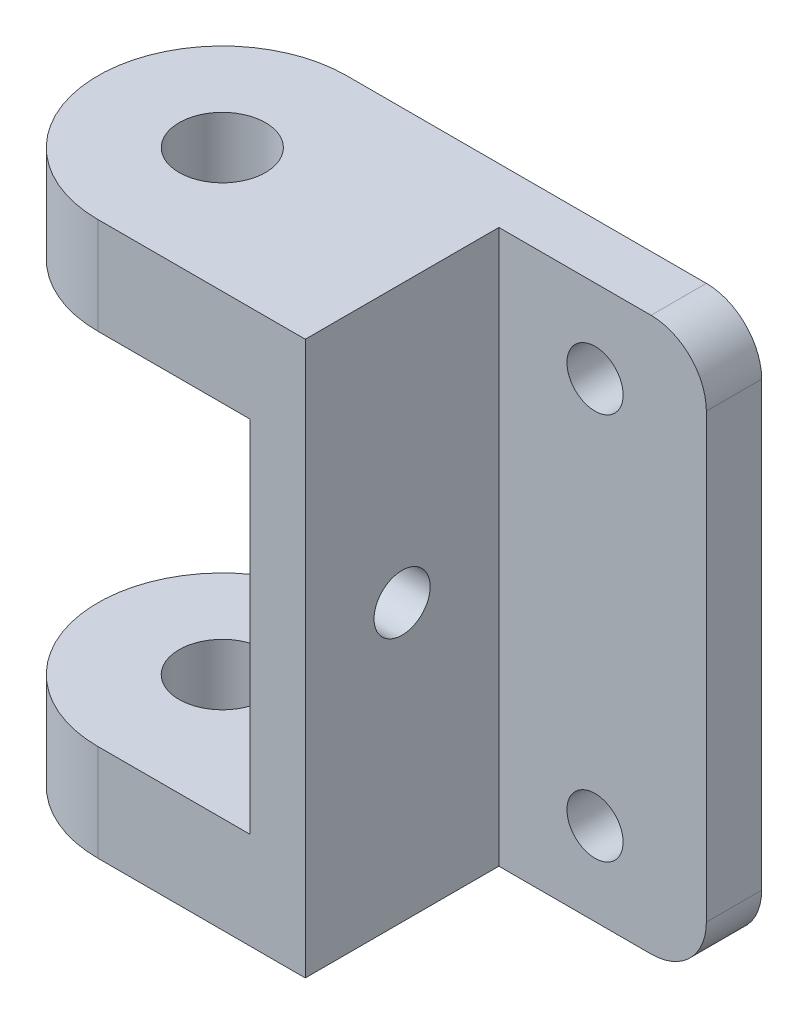
ISO-10303-21;
HEADER;
FILE_DESCRIPTION(('STEP AP214'),'2;1');
FILE_NAME('part.step','',(''),(''),'','','');
FILE_SCHEMA(('AUTOMOTIVE_DESIGN { 1 0 10303 214 1 1 1 1 }'));
ENDSEC;
DATA;
#1=APPLICATION_CONTEXT('core data for automotive mechanical design processes');
#2=APPLICATION_PROTOCOL_DEFINITION('international standard','automotive_design',2000,#1);
#3=PRODUCT_CONTEXT('',#1,'mechanical');
#4=PRODUCT('Part','Part','',(#3));
#5=PRODUCT_RELATED_PRODUCT_CATEGORY('part','',(#4));
#6=PRODUCT_DEFINITION_FORMATION('','',#4);
#7=PRODUCT_DEFINITION_CONTEXT('part definition',#1,'design');
#8=PRODUCT_DEFINITION('design','',#6,#7);
#9=PRODUCT_DEFINITION_SHAPE('','',#8);
#10=(LENGTH_UNIT() NAMED_UNIT(*) SI_UNIT(.MILLI.,.METRE.));
#11=(NAMED_UNIT(*) PLANE_ANGLE_UNIT() SI_UNIT($,.RADIAN.));
#12=(NAMED_UNIT(*) SI_UNIT($,.STERADIAN.) SOLID_ANGLE_UNIT());
#13=UNCERTAINTY_MEASURE_WITH_UNIT(LENGTH_MEASURE(1.E-05),#10,'distance_accuracy_value','');
#14=(GEOMETRIC_REPRESENTATION_CONTEXT(3) GLOBAL_UNCERTAINTY_ASSIGNED_CONTEXT((#13)) GLOBAL_UNIT_ASSIGNED_CONTEXT((#10,
#11,#12)) REPRESENTATION_CONTEXT('',''));
#15=CARTESIAN_POINT('',(0.,0.,0.));
#16=DIRECTION('',(0.,0.,1.));
#17=DIRECTION('',(1.,0.,0.));
#18=AXIS2_PLACEMENT_3D('',#15,#16,#17);
#19=CARTESIAN_POINT('',(0.,-0.7,0.9));
#20=DIRECTION('',(0.,1.,0.));
#21=DIRECTION('',(0.,0.,1.));
#22=AXIS2_PLACEMENT_3D('',#19,#20,#21);
#23=PLANE('',#22);
#24=CARTESIAN_POINT('',(0.,-0.7,0.9));
#25=DIRECTION('',(0.,1.,0.));
#26=DIRECTION('',(0.,0.,1.));
#27=AXIS2_PLACEMENT_3D('',#24,#25,#26);
#28=CIRCLE('',#27,0.3125);
#29=CARTESIAN_POINT('',(0.,-0.7,1.2125));
#30=VERTEX_POINT('',#29);
#31=EDGE_CURVE('E258',#30,#30,#28,.T.);
#32=ORIENTED_EDGE('',*,*,#31,.T.);
#33=EDGE_LOOP('',(#32));
#34=FACE_BOUND('',#33,.T.);
#35=DIRECTION('',(0.,0.,-1.));
#36=VECTOR('',#35,1.);
#37=CARTESIAN_POINT('',(1.1,-0.7,0.));
#38=LINE('',#37,#36);
#39=CARTESIAN_POINT('',(1.1,-0.7,1.8));
#40=VERTEX_POINT('',#39);
#41=CARTESIAN_POINT('',(1.1,-0.7,0.));
#42=VERTEX_POINT('',#41);
#43=EDGE_CURVE('E143',#40,#42,#38,.T.);
#44=ORIENTED_EDGE('',*,*,#43,.F.);
#45=DIRECTION('',(1.,0.,0.));
#46=VECTOR('',#45,1.);
#47=CARTESIAN_POINT('',(0.,-0.7,1.8));
#48=LINE('',#47,#46);
#49=CARTESIAN_POINT('',(0.,-0.7,1.8));
#50=VERTEX_POINT('',#49);
#51=EDGE_CURVE('E183',#50,#40,#48,.T.);
#52=ORIENTED_EDGE('',*,*,#51,.F.);
#53=CARTESIAN_POINT('',(0.,-0.7,0.9));
#54=DIRECTION('',(0.,1.,0.));
#55=DIRECTION('',(0.,0.,1.));
#56=AXIS2_PLACEMENT_3D('',#53,#54,#55);
#57=CIRCLE('',#56,0.9);
#58=CARTESIAN_POINT('',(0.,-0.7,0.));
#59=VERTEX_POINT('',#58);
#60=EDGE_CURVE('E181',#59,#50,#57,.T.);
#61=ORIENTED_EDGE('',*,*,#60,.F.);
#62=DIRECTION('',(-1.,0.,0.));
#63=VECTOR('',#62,1.);
#64=CARTESIAN_POINT('',(1.5,-0.7,0.));
#65=LINE('',#64,#63);
#66=EDGE_CURVE('E189',#42,#59,#65,.T.);
#67=ORIENTED_EDGE('',*,*,#66,.F.);
#68=EDGE_LOOP('',(#44,#52,#61,#67));
#69=FACE_BOUND('',#68,.T.);
#70=ADVANCED_FACE('F50',(#34,#69),#23,.F.);
#71=CARTESIAN_POINT('',(0.,-3.3,0.9));
#72=DIRECTION('',(0.,-1.,0.));
#73=DIRECTION('',(0.,0.,-1.));
#74=AXIS2_PLACEMENT_3D('',#71,#72,#73);
#75=PLANE('',#74);
#76=CARTESIAN_POINT('',(0.,-3.3,0.9));
#77=DIRECTION('',(0.,-1.,0.));
#78=DIRECTION('',(0.,0.,-1.));
#79=AXIS2_PLACEMENT_3D('',#76,#77,#78);
#80=CIRCLE('',#79,0.3125);
#81=CARTESIAN_POINT('',(0.,-3.3,0.5875));
#82=VERTEX_POINT('',#81);
#83=EDGE_CURVE('E272',#82,#82,#80,.T.);
#84=ORIENTED_EDGE('',*,*,#83,.T.);
#85=EDGE_LOOP('',(#84));
#86=FACE_BOUND('',#85,.T.);
#87=DIRECTION('',(0.,0.,1.));
#88=VECTOR('',#87,1.);
#89=CARTESIAN_POINT('',(1.1,-3.3,1.8));
#90=LINE('',#89,#88);
#91=CARTESIAN_POINT('',(1.1,-3.3,0.));
#92=VERTEX_POINT('',#91);
#93=CARTESIAN_POINT('',(1.1,-3.3,1.8));
#94=VERTEX_POINT('',#93);
#95=EDGE_CURVE('E145',#92,#94,#90,.T.);
#96=ORIENTED_EDGE('',*,*,#95,.F.);
#97=DIRECTION('',(1.,0.,0.));
#98=VECTOR('',#97,1.);
#99=CARTESIAN_POINT('',(1.5,-3.3,0.));
#100=LINE('',#99,#98);
#101=CARTESIAN_POINT('',(0.,-3.3,0.));
#102=VERTEX_POINT('',#101);
#103=EDGE_CURVE('E153',#102,#92,#100,.T.);
#104=ORIENTED_EDGE('',*,*,#103,.F.);
#105=CARTESIAN_POINT('',(0.,-3.3,0.9));
#106=DIRECTION('',(0.,-1.,0.));
#107=DIRECTION('',(0.,0.,-1.));
#108=AXIS2_PLACEMENT_3D('',#105,#106,#107);
#109=CIRCLE('',#108,0.9);
#110=CARTESIAN_POINT('',(0.,-3.3,1.8));
#111=VERTEX_POINT('',#110);
#112=EDGE_CURVE('E165',#111,#102,#109,.T.);
#113=ORIENTED_EDGE('',*,*,#112,.F.);
#114=DIRECTION('',(-1.,0.,0.));
#115=VECTOR('',#114,1.);
#116=CARTESIAN_POINT('',(0.,-3.3,1.8));
#117=LINE('',#116,#115);
#118=EDGE_CURVE('E157',#94,#111,#117,.T.);
#119=ORIENTED_EDGE('',*,*,#118,.F.);
#120=EDGE_LOOP('',(#96,#104,#113,#119));
#121=FACE_BOUND('',#120,.T.);
#122=ADVANCED_FACE('F154',(#86,#121),#75,.F.);
#123=CARTESIAN_POINT('',(2.6,-3.6,0.4));
#124=DIRECTION('',(0.,0.,-1.));
#125=DIRECTION('',(-1.,0.,0.));
#126=AXIS2_PLACEMENT_3D('',#123,#124,#125);
#127=CYLINDRICAL_SURFACE('',#126,0.4);
#128=CARTESIAN_POINT('',(2.6,-3.6,0.));
#129=DIRECTION('',(0.,0.,1.));
#130=DIRECTION('',(1.,0.,0.));
#131=AXIS2_PLACEMENT_3D('',#128,#129,#130);
#132=CIRCLE('',#131,0.4);
#133=CARTESIAN_POINT('',(3.,-3.6,0.));
#134=VERTEX_POINT('',#133);
#135=CARTESIAN_POINT('',(2.6,-4.,0.));
#136=VERTEX_POINT('',#135);
#137=EDGE_CURVE('E203',#134,#136,#132,.F.);
#138=ORIENTED_EDGE('',*,*,#137,.F.);
#139=DIRECTION('',(0.,0.,-1.));
#140=VECTOR('',#139,1.);
#141=CARTESIAN_POINT('',(3.,-3.6,0.4));
#142=LINE('',#141,#140);
#143=CARTESIAN_POINT('',(3.,-3.6,0.4));
#144=VERTEX_POINT('',#143);
#145=EDGE_CURVE('E11',#144,#134,#142,.T.);
#146=ORIENTED_EDGE('',*,*,#145,.F.);
#147=CARTESIAN_POINT('',(2.6,-3.6,0.4));
#148=DIRECTION('',(0.,0.,1.));
#149=DIRECTION('',(1.,0.,0.));
#150=AXIS2_PLACEMENT_3D('',#147,#148,#149);
#151=CIRCLE('',#150,0.4);
#152=CARTESIAN_POINT('',(2.6,-4.,0.4));
#153=VERTEX_POINT('',#152);
#154=EDGE_CURVE('E207',#144,#153,#151,.F.);
#155=ORIENTED_EDGE('',*,*,#154,.T.);
#156=DIRECTION('',(0.,0.,-1.));
#157=VECTOR('',#156,1.);
#158=CARTESIAN_POINT('',(2.6,-4.,0.4));
#159=LINE('',#158,#157);
#160=EDGE_CURVE('E61',#153,#136,#159,.T.);
#161=ORIENTED_EDGE('',*,*,#160,.T.);
#162=EDGE_LOOP('',(#138,#146,#155,#161));
#163=FACE_BOUND('',#162,.T.);
#164=ADVANCED_FACE('F47',(#163),#127,.T.);
#165=CARTESIAN_POINT('',(3.,0.,0.4));
#166=DIRECTION('',(1.,0.,0.));
#167=DIRECTION('',(0.,0.,-1.));
#168=AXIS2_PLACEMENT_3D('',#165,#166,#167);
#169=PLANE('',#168);
#170=DIRECTION('',(0.,-1.,0.));
#171=VECTOR('',#170,1.);
#172=CARTESIAN_POINT('',(3.,0.,0.));
#173=LINE('',#172,#171);
#174=CARTESIAN_POINT('',(3.,-0.400000000000003,0.));
#175=VERTEX_POINT('',#174);
#176=EDGE_CURVE('E218',#175,#134,#173,.T.);
#177=ORIENTED_EDGE('',*,*,#176,.F.);
#178=DIRECTION('',(0.,0.,-1.));
#179=VECTOR('',#178,1.);
#180=CARTESIAN_POINT('',(3.,-0.400000000000003,0.4));
#181=LINE('',#180,#179);
#182=CARTESIAN_POINT('',(3.,-0.400000000000003,0.4));
#183=VERTEX_POINT('',#182);
#184=EDGE_CURVE('E57',#183,#175,#181,.T.);
#185=ORIENTED_EDGE('',*,*,#184,.F.);
#186=DIRECTION('',(0.,-1.,0.));
#187=VECTOR('',#186,1.);
#188=CARTESIAN_POINT('',(3.,0.,0.4));
#189=LINE('',#188,#187);
#190=EDGE_CURVE('E206',#183,#144,#189,.T.);
#191=ORIENTED_EDGE('',*,*,#190,.T.);
#192=ORIENTED_EDGE('',*,*,#145,.T.);
#193=EDGE_LOOP('',(#177,#185,#191,#192));
#194=FACE_BOUND('',#193,.T.);
#195=ADVANCED_FACE('F240',(#194),#169,.T.);
#196=CARTESIAN_POINT('',(2.6,-0.4,0.4));
#197=DIRECTION('',(0.,0.,-1.));
#198=DIRECTION('',(-1.,0.,0.));
#199=AXIS2_PLACEMENT_3D('',#196,#197,#198);
#200=CYLINDRICAL_SURFACE('',#199,0.4);
#201=CARTESIAN_POINT('',(2.6,-0.4,0.));
#202=DIRECTION('',(0.,0.,1.));
#203=DIRECTION('',(1.,0.,0.));
#204=AXIS2_PLACEMENT_3D('',#201,#202,#203);
#205=CIRCLE('',#204,0.4);
#206=CARTESIAN_POINT('',(2.6,0.,0.));
#207=VERTEX_POINT('',#206);
#208=EDGE_CURVE('E225',#175,#207,#205,.T.);
#209=ORIENTED_EDGE('',*,*,#208,.T.);
#210=DIRECTION('',(0.,0.,-1.));
#211=VECTOR('',#210,1.);
#212=CARTESIAN_POINT('',(2.6,0.,0.4));
#213=LINE('',#212,#211);
#214=CARTESIAN_POINT('',(2.6,0.,0.4));
#215=VERTEX_POINT('',#214);
#216=EDGE_CURVE('E230',#215,#207,#213,.T.);
#217=ORIENTED_EDGE('',*,*,#216,.F.);
#218=CARTESIAN_POINT('',(2.6,-0.4,0.4));
#219=DIRECTION('',(0.,0.,1.));
#220=DIRECTION('',(1.,0.,0.));
#221=AXIS2_PLACEMENT_3D('',#218,#219,#220);
#222=CIRCLE('',#221,0.4);
#223=EDGE_CURVE('E215',#183,#215,#222,.T.);
#224=ORIENTED_EDGE('',*,*,#223,.F.);
#225=ORIENTED_EDGE('',*,*,#184,.T.);
#226=EDGE_LOOP('',(#209,#217,#224,#225));
#227=FACE_BOUND('',#226,.T.);
#228=ADVANCED_FACE('F235',(#227),#200,.T.);
#229=CARTESIAN_POINT('',(0.,0.,0.4));
#230=DIRECTION('',(0.,1.,0.));
#231=DIRECTION('',(0.,0.,1.));
#232=AXIS2_PLACEMENT_3D('',#229,#230,#231);
#233=PLANE('',#232);
#234=CARTESIAN_POINT('',(0.,0.,0.9));
#235=DIRECTION('',(0.,1.,0.));
#236=DIRECTION('',(0.,0.,1.));
#237=AXIS2_PLACEMENT_3D('',#234,#235,#236);
#238=CIRCLE('',#237,0.3125);
#239=CARTESIAN_POINT('',(0.,0.,1.2125));
#240=VERTEX_POINT('',#239);
#241=EDGE_CURVE('E270',#240,#240,#238,.T.);
#242=ORIENTED_EDGE('',*,*,#241,.F.);
#243=EDGE_LOOP('',(#242));
#244=FACE_BOUND('',#243,.T.);
#245=DIRECTION('',(1.,0.,0.));
#246=VECTOR('',#245,1.);
#247=CARTESIAN_POINT('',(0.,0.,0.));
#248=LINE('',#247,#246);
#249=CARTESIAN_POINT('',(0.,0.,0.));
#250=VERTEX_POINT('',#249);
#251=EDGE_CURVE('E85',#250,#207,#248,.T.);
#252=ORIENTED_EDGE('',*,*,#251,.F.);
#253=CARTESIAN_POINT('',(0.,0.,0.9));
#254=DIRECTION('',(0.,1.,0.));
#255=DIRECTION('',(0.,0.,1.));
#256=AXIS2_PLACEMENT_3D('',#253,#254,#255);
#257=CIRCLE('',#256,0.9);
#258=CARTESIAN_POINT('',(0.,0.,1.8));
#259=VERTEX_POINT('',#258);
#260=EDGE_CURVE('E177',#250,#259,#257,.T.);
#261=ORIENTED_EDGE('',*,*,#260,.T.);
#262=DIRECTION('',(1.,0.,0.));
#263=VECTOR('',#262,1.);
#264=CARTESIAN_POINT('',(0.,0.,1.8));
#265=LINE('',#264,#263);
#266=CARTESIAN_POINT('',(1.5,0.,1.8));
#267=VERTEX_POINT('',#266);
#268=EDGE_CURVE('E194',#259,#267,#265,.T.);
#269=ORIENTED_EDGE('',*,*,#268,.T.);
#270=DIRECTION('',(0.,0.,-1.));
#271=VECTOR('',#270,1.);
#272=CARTESIAN_POINT('',(1.5,0.,1.8));
#273=LINE('',#272,#271);
#274=CARTESIAN_POINT('',(1.5,0.,0.4));
#275=VERTEX_POINT('',#274);
#276=EDGE_CURVE('E184',#267,#275,#273,.T.);
#277=ORIENTED_EDGE('',*,*,#276,.T.);
#278=DIRECTION('',(1.,0.,0.));
#279=VECTOR('',#278,1.);
#280=CARTESIAN_POINT('',(0.,0.,0.4));
#281=LINE('',#280,#279);
#282=EDGE_CURVE('E213',#275,#215,#281,.T.);
#283=ORIENTED_EDGE('',*,*,#282,.T.);
#284=ORIENTED_EDGE('',*,*,#216,.T.);
#285=EDGE_LOOP('',(#252,#261,#269,#277,#283,#284));
#286=FACE_BOUND('',#285,.T.);
#287=ADVANCED_FACE('F288',(#244,#286),#233,.T.);
#288=CARTESIAN_POINT('',(0.,-4.,0.4));
#289=DIRECTION('',(0.,-1.,0.));
#290=DIRECTION('',(0.,0.,-1.));
#291=AXIS2_PLACEMENT_3D('',#288,#289,#290);
#292=PLANE('',#291);
#293=CARTESIAN_POINT('',(0.,-4.,0.9));
#294=DIRECTION('',(0.,-1.,0.));
#295=DIRECTION('',(0.,0.,-1.));
#296=AXIS2_PLACEMENT_3D('',#293,#294,#295);
#297=CIRCLE('',#296,0.3125);
#298=CARTESIAN_POINT('',(0.,-4.,0.5875));
#299=VERTEX_POINT('',#298);
#300=EDGE_CURVE('E274',#299,#299,#297,.T.);
#301=ORIENTED_EDGE('',*,*,#300,.F.);
#302=EDGE_LOOP('',(#301));
#303=FACE_BOUND('',#302,.T.);
#304=DIRECTION('',(-1.,0.,0.));
#305=VECTOR('',#304,1.);
#306=CARTESIAN_POINT('',(0.,-4.,0.4));
#307=LINE('',#306,#305);
#308=CARTESIAN_POINT('',(1.5,-4.,0.4));
#309=VERTEX_POINT('',#308);
#310=EDGE_CURVE('E220',#153,#309,#307,.T.);
#311=ORIENTED_EDGE('',*,*,#310,.T.);
#312=DIRECTION('',(0.,0.,1.));
#313=VECTOR('',#312,1.);
#314=CARTESIAN_POINT('',(1.5,-4.,1.8));
#315=LINE('',#314,#313);
#316=CARTESIAN_POINT('',(1.5,-4.,1.8));
#317=VERTEX_POINT('',#316);
#318=EDGE_CURVE('E167',#309,#317,#315,.T.);
#319=ORIENTED_EDGE('',*,*,#318,.T.);
#320=DIRECTION('',(-1.,0.,0.));
#321=VECTOR('',#320,1.);
#322=CARTESIAN_POINT('',(0.,-4.,1.8));
#323=LINE('',#322,#321);
#324=CARTESIAN_POINT('',(0.,-4.,1.8));
#325=VERTEX_POINT('',#324);
#326=EDGE_CURVE('E173',#317,#325,#323,.T.);
#327=ORIENTED_EDGE('',*,*,#326,.T.);
#328=CARTESIAN_POINT('',(0.,-4.,0.9));
#329=DIRECTION('',(0.,-1.,0.));
#330=DIRECTION('',(0.,0.,-1.));
#331=AXIS2_PLACEMENT_3D('',#328,#329,#330);
#332=CIRCLE('',#331,0.9);
#333=CARTESIAN_POINT('',(0.,-4.,0.));
#334=VERTEX_POINT('',#333);
#335=EDGE_CURVE('E176',#325,#334,#332,.T.);
#336=ORIENTED_EDGE('',*,*,#335,.T.);
#337=DIRECTION('',(-1.,0.,0.));
#338=VECTOR('',#337,1.);
#339=CARTESIAN_POINT('',(0.,-4.,0.));
#340=LINE('',#339,#338);
#341=EDGE_CURVE('E209',#136,#334,#340,.T.);
#342=ORIENTED_EDGE('',*,*,#341,.F.);
#343=ORIENTED_EDGE('',*,*,#160,.F.);
#344=EDGE_LOOP('',(#311,#319,#327,#336,#342,#343));
#345=FACE_BOUND('',#344,.T.);
#346=ADVANCED_FACE('F238',(#303,#345),#292,.T.);
#347=CARTESIAN_POINT('',(0.,0.,0.4));
#348=DIRECTION('',(0.,0.,1.));
#349=DIRECTION('',(1.,0.,0.));
#350=AXIS2_PLACEMENT_3D('',#347,#348,#349);
#351=PLANE('',#350);
#352=CARTESIAN_POINT('',(2.195,-0.6,0.4));
#353=DIRECTION('',(0.,0.,1.));
#354=DIRECTION('',(1.,0.,0.));
#355=AXIS2_PLACEMENT_3D('',#352,#353,#354);
#356=CIRCLE('',#355,0.203);
#357=CARTESIAN_POINT('',(2.398,-0.6,0.4));
#358=VERTEX_POINT('',#357);
#359=EDGE_CURVE('E264',#358,#358,#356,.T.);
#360=ORIENTED_EDGE('',*,*,#359,.F.);
#361=EDGE_LOOP('',(#360));
#362=FACE_BOUND('',#361,.T.);
#363=CARTESIAN_POINT('',(2.195,-3.4,0.4));
#364=DIRECTION('',(0.,0.,1.));
#365=DIRECTION('',(1.,0.,0.));
#366=AXIS2_PLACEMENT_3D('',#363,#364,#365);
#367=CIRCLE('',#366,0.203);
#368=CARTESIAN_POINT('',(2.398,-3.4,0.4));
#369=VERTEX_POINT('',#368);
#370=EDGE_CURVE('E257',#369,#369,#367,.T.);
#371=ORIENTED_EDGE('',*,*,#370,.F.);
#372=EDGE_LOOP('',(#371));
#373=FACE_BOUND('',#372,.T.);
#374=DIRECTION('',(0.,1.,0.));
#375=VECTOR('',#374,1.);
#376=CARTESIAN_POINT('',(1.5,0.,0.4));
#377=LINE('',#376,#375);
#378=EDGE_CURVE('E198',#309,#275,#377,.T.);
#379=ORIENTED_EDGE('',*,*,#378,.F.);
#380=ORIENTED_EDGE('',*,*,#310,.F.);
#381=ORIENTED_EDGE('',*,*,#154,.F.);
#382=ORIENTED_EDGE('',*,*,#190,.F.);
#383=ORIENTED_EDGE('',*,*,#223,.T.);
#384=ORIENTED_EDGE('',*,*,#282,.F.);
#385=EDGE_LOOP('',(#379,#380,#381,#382,#383,#384));
#386=FACE_BOUND('',#385,.T.);
#387=ADVANCED_FACE('F286',(#362,#373,#386),#351,.T.);
#388=CARTESIAN_POINT('',(0.,0.,0.));
#389=DIRECTION('',(0.,0.,1.));
#390=DIRECTION('',(1.,0.,0.));
#391=AXIS2_PLACEMENT_3D('',#388,#389,#390);
#392=PLANE('',#391);
#393=CARTESIAN_POINT('',(2.195,-0.6,0.));
#394=DIRECTION('',(0.,0.,1.));
#395=DIRECTION('',(1.,0.,0.));
#396=AXIS2_PLACEMENT_3D('',#393,#394,#395);
#397=CIRCLE('',#396,0.203);
#398=CARTESIAN_POINT('',(2.398,-0.6,0.));
#399=VERTEX_POINT('',#398);
#400=EDGE_CURVE('E254',#399,#399,#397,.T.);
#401=ORIENTED_EDGE('',*,*,#400,.T.);
#402=EDGE_LOOP('',(#401));
#403=FACE_BOUND('',#402,.T.);
#404=CARTESIAN_POINT('',(2.195,-3.4,0.));
#405=DIRECTION('',(0.,0.,1.));
#406=DIRECTION('',(1.,0.,0.));
#407=AXIS2_PLACEMENT_3D('',#404,#405,#406);
#408=CIRCLE('',#407,0.203);
#409=CARTESIAN_POINT('',(2.398,-3.4,0.));
#410=VERTEX_POINT('',#409);
#411=EDGE_CURVE('E256',#410,#410,#408,.T.);
#412=ORIENTED_EDGE('',*,*,#411,.T.);
#413=EDGE_LOOP('',(#412));
#414=FACE_BOUND('',#413,.T.);
#415=DIRECTION('',(0.,-1.,0.));
#416=VECTOR('',#415,1.);
#417=CARTESIAN_POINT('',(1.1,-3.3,0.));
#418=LINE('',#417,#416);
#419=EDGE_CURVE('E136',#42,#92,#418,.T.);
#420=ORIENTED_EDGE('',*,*,#419,.F.);
#421=ORIENTED_EDGE('',*,*,#66,.T.);
#422=DIRECTION('',(0.,1.,0.));
#423=VECTOR('',#422,1.);
#424=CARTESIAN_POINT('',(0.,-0.7,0.));
#425=LINE('',#424,#423);
#426=EDGE_CURVE('E199',#59,#250,#425,.T.);
#427=ORIENTED_EDGE('',*,*,#426,.T.);
#428=ORIENTED_EDGE('',*,*,#251,.T.);
#429=ORIENTED_EDGE('',*,*,#208,.F.);
#430=ORIENTED_EDGE('',*,*,#176,.T.);
#431=ORIENTED_EDGE('',*,*,#137,.T.);
#432=ORIENTED_EDGE('',*,*,#341,.T.);
#433=DIRECTION('',(0.,-1.,0.));
#434=VECTOR('',#433,1.);
#435=CARTESIAN_POINT('',(0.,-3.3,0.));
#436=LINE('',#435,#434);
#437=EDGE_CURVE('E163',#102,#334,#436,.T.);
#438=ORIENTED_EDGE('',*,*,#437,.F.);
#439=ORIENTED_EDGE('',*,*,#103,.T.);
#440=EDGE_LOOP('',(#420,#421,#427,#428,#429,#430,#431,#432,#438,#439));
#441=FACE_BOUND('',#440,.T.);
#442=ADVANCED_FACE('F156',(#403,#414,#441),#392,.F.);
#443=CARTESIAN_POINT('',(0.,-0.7,0.9));
#444=DIRECTION('',(0.,1.,0.));
#445=DIRECTION('',(0.,0.,1.));
#446=AXIS2_PLACEMENT_3D('',#443,#444,#445);
#447=CYLINDRICAL_SURFACE('',#446,0.9);
#448=ORIENTED_EDGE('',*,*,#260,.F.);
#449=ORIENTED_EDGE('',*,*,#426,.F.);
#450=ORIENTED_EDGE('',*,*,#60,.T.);
#451=DIRECTION('',(0.,1.,0.));
#452=VECTOR('',#451,1.);
#453=CARTESIAN_POINT('',(0.,-0.7,1.8));
#454=LINE('',#453,#452);
#455=EDGE_CURVE('E188',#50,#259,#454,.T.);
#456=ORIENTED_EDGE('',*,*,#455,.T.);
#457=EDGE_LOOP('',(#448,#449,#450,#456));
#458=FACE_BOUND('',#457,.T.);
#459=ADVANCED_FACE('F317',(#458),#447,.T.);
#460=CARTESIAN_POINT('',(1.5,-0.7,1.8));
#461=DIRECTION('',(1.,0.,0.));
#462=DIRECTION('',(0.,0.,-1.));
#463=AXIS2_PLACEMENT_3D('',#460,#461,#462);
#464=PLANE('',#463);
#465=CARTESIAN_POINT('',(1.5,-2.,1.1));
#466=DIRECTION('',(1.,0.,0.));
#467=DIRECTION('',(0.,0.,-1.));
#468=AXIS2_PLACEMENT_3D('',#465,#466,#467);
#469=CIRCLE('',#468,0.203);
#470=CARTESIAN_POINT('',(1.5,-2.,0.897));
#471=VERTEX_POINT('',#470);
#472=EDGE_CURVE('E249',#471,#471,#469,.T.);
#473=ORIENTED_EDGE('',*,*,#472,.F.);
#474=EDGE_LOOP('',(#473));
#475=FACE_BOUND('',#474,.T.);
#476=DIRECTION('',(0.,1.,0.));
#477=VECTOR('',#476,1.);
#478=CARTESIAN_POINT('',(1.5,-0.7,1.8));
#479=LINE('',#478,#477);
#480=EDGE_CURVE('E202',#317,#267,#479,.T.);
#481=ORIENTED_EDGE('',*,*,#480,.F.);
#482=ORIENTED_EDGE('',*,*,#318,.F.);
#483=ORIENTED_EDGE('',*,*,#378,.T.);
#484=ORIENTED_EDGE('',*,*,#276,.F.);
#485=EDGE_LOOP('',(#481,#482,#483,#484));
#486=FACE_BOUND('',#485,.T.);
#487=ADVANCED_FACE('F312',(#475,#486),#464,.T.);
#488=CARTESIAN_POINT('',(0.,-0.7,1.8));
#489=DIRECTION('',(0.,0.,1.));
#490=DIRECTION('',(1.,0.,0.));
#491=AXIS2_PLACEMENT_3D('',#488,#489,#490);
#492=PLANE('',#491);
#493=ORIENTED_EDGE('',*,*,#268,.F.);
#494=ORIENTED_EDGE('',*,*,#455,.F.);
#495=ORIENTED_EDGE('',*,*,#51,.T.);
#496=DIRECTION('',(0.,1.,0.));
#497=VECTOR('',#496,1.);
#498=CARTESIAN_POINT('',(1.1,-0.7,1.8));
#499=LINE('',#498,#497);
#500=EDGE_CURVE('E159',#94,#40,#499,.T.);
#501=ORIENTED_EDGE('',*,*,#500,.F.);
#502=ORIENTED_EDGE('',*,*,#118,.T.);
#503=DIRECTION('',(0.,-1.,0.));
#504=VECTOR('',#503,1.);
#505=CARTESIAN_POINT('',(0.,-3.3,1.8));
#506=LINE('',#505,#504);
#507=EDGE_CURVE('E161',#111,#325,#506,.T.);
#508=ORIENTED_EDGE('',*,*,#507,.T.);
#509=ORIENTED_EDGE('',*,*,#326,.F.);
#510=ORIENTED_EDGE('',*,*,#480,.T.);
#511=EDGE_LOOP('',(#493,#494,#495,#501,#502,#508,#509,#510));
#512=FACE_BOUND('',#511,.T.);
#513=ADVANCED_FACE('F246',(#512),#492,.T.);
#514=CARTESIAN_POINT('',(0.,-3.3,0.9));
#515=DIRECTION('',(0.,-1.,0.));
#516=DIRECTION('',(0.,0.,-1.));
#517=AXIS2_PLACEMENT_3D('',#514,#515,#516);
#518=CYLINDRICAL_SURFACE('',#517,0.9);
#519=ORIENTED_EDGE('',*,*,#335,.F.);
#520=ORIENTED_EDGE('',*,*,#507,.F.);
#521=ORIENTED_EDGE('',*,*,#112,.T.);
#522=ORIENTED_EDGE('',*,*,#437,.T.);
#523=EDGE_LOOP('',(#519,#520,#521,#522));
#524=FACE_BOUND('',#523,.T.);
#525=ADVANCED_FACE('F243',(#524),#518,.T.);
#526=CARTESIAN_POINT('',(1.1,0.,0.));
#527=DIRECTION('',(1.,0.,0.));
#528=DIRECTION('',(0.,0.,-1.));
#529=AXIS2_PLACEMENT_3D('',#526,#527,#528);
#530=PLANE('',#529);
#531=CARTESIAN_POINT('',(1.1,-2.,1.1));
#532=DIRECTION('',(1.,0.,0.));
#533=DIRECTION('',(0.,0.,-1.));
#534=AXIS2_PLACEMENT_3D('',#531,#532,#533);
#535=CIRCLE('',#534,0.203);
#536=CARTESIAN_POINT('',(1.1,-2.,0.897));
#537=VERTEX_POINT('',#536);
#538=EDGE_CURVE('E149',#537,#537,#535,.T.);
#539=ORIENTED_EDGE('',*,*,#538,.T.);
#540=EDGE_LOOP('',(#539));
#541=FACE_BOUND('',#540,.T.);
#542=ORIENTED_EDGE('',*,*,#419,.T.);
#543=ORIENTED_EDGE('',*,*,#95,.T.);
#544=ORIENTED_EDGE('',*,*,#500,.T.);
#545=ORIENTED_EDGE('',*,*,#43,.T.);
#546=EDGE_LOOP('',(#542,#543,#544,#545));
#547=FACE_BOUND('',#546,.T.);
#548=ADVANCED_FACE('F142',(#541,#547),#530,.F.);
#549=CARTESIAN_POINT('',(1.1,-2.,1.1));
#550=DIRECTION('',(1.,0.,0.));
#551=DIRECTION('',(0.,0.,-1.));
#552=AXIS2_PLACEMENT_3D('',#549,#550,#551);
#553=CYLINDRICAL_SURFACE('',#552,0.203);
#554=ORIENTED_EDGE('',*,*,#538,.F.);
#555=EDGE_LOOP('',(#554));
#556=FACE_BOUND('',#555,.T.);
#557=ORIENTED_EDGE('',*,*,#472,.T.);
#558=EDGE_LOOP('',(#557));
#559=FACE_BOUND('',#558,.T.);
#560=ADVANCED_FACE('F331',(#556,#559),#553,.F.);
#561=CARTESIAN_POINT('',(2.195,-3.4,0.));
#562=DIRECTION('',(0.,0.,1.));
#563=DIRECTION('',(1.,0.,0.));
#564=AXIS2_PLACEMENT_3D('',#561,#562,#563);
#565=CYLINDRICAL_SURFACE('',#564,0.203);
#566=ORIENTED_EDGE('',*,*,#411,.F.);
#567=EDGE_LOOP('',(#566));
#568=FACE_BOUND('',#567,.T.);
#569=ORIENTED_EDGE('',*,*,#370,.T.);
#570=EDGE_LOOP('',(#569));
#571=FACE_BOUND('',#570,.T.);
#572=ADVANCED_FACE('F328',(#568,#571),#565,.F.);
#573=CARTESIAN_POINT('',(2.195,-0.6,0.));
#574=DIRECTION('',(0.,0.,1.));
#575=DIRECTION('',(1.,0.,0.));
#576=AXIS2_PLACEMENT_3D('',#573,#574,#575);
#577=CYLINDRICAL_SURFACE('',#576,0.203);
#578=ORIENTED_EDGE('',*,*,#400,.F.);
#579=EDGE_LOOP('',(#578));
#580=FACE_BOUND('',#579,.T.);
#581=ORIENTED_EDGE('',*,*,#359,.T.);
#582=EDGE_LOOP('',(#581));
#583=FACE_BOUND('',#582,.T.);
#584=ADVANCED_FACE('F335',(#580,#583),#577,.F.);
#585=CARTESIAN_POINT('',(0.,-0.7,0.9));
#586=DIRECTION('',(0.,1.,0.));
#587=DIRECTION('',(0.,0.,1.));
#588=AXIS2_PLACEMENT_3D('',#585,#586,#587);
#589=CYLINDRICAL_SURFACE('',#588,0.3125);
#590=ORIENTED_EDGE('',*,*,#31,.F.);
#591=EDGE_LOOP('',(#590));
#592=FACE_BOUND('',#591,.T.);
#593=ORIENTED_EDGE('',*,*,#241,.T.);
#594=EDGE_LOOP('',(#593));
#595=FACE_BOUND('',#594,.T.);
#596=ADVANCED_FACE('F281',(#592,#595),#589,.F.);
#597=CARTESIAN_POINT('',(0.,-3.3,0.9));
#598=DIRECTION('',(0.,-1.,0.));
#599=DIRECTION('',(0.,0.,-1.));
#600=AXIS2_PLACEMENT_3D('',#597,#598,#599);
#601=CYLINDRICAL_SURFACE('',#600,0.3125);
#602=ORIENTED_EDGE('',*,*,#83,.F.);
#603=EDGE_LOOP('',(#602));
#604=FACE_BOUND('',#603,.T.);
#605=ORIENTED_EDGE('',*,*,#300,.T.);
#606=EDGE_LOOP('',(#605));
#607=FACE_BOUND('',#606,.T.);
#608=ADVANCED_FACE('F282',(#604,#607),#601,.F.);
#609=CLOSED_SHELL('',(#70,#122,#164,#195,#228,#287,#346,#387,#442,#459,#487,#513,#525,#548,#560,
#572,#584,#596,#608));
#610=MANIFOLD_SOLID_BREP('B2',#609);
#611=ADVANCED_BREP_SHAPE_REPRESENTATION('',(#18,#610),#14);
#612=SHAPE_DEFINITION_REPRESENTATION(#9,#611);
ENDSEC;
END-ISO-10303-21;
